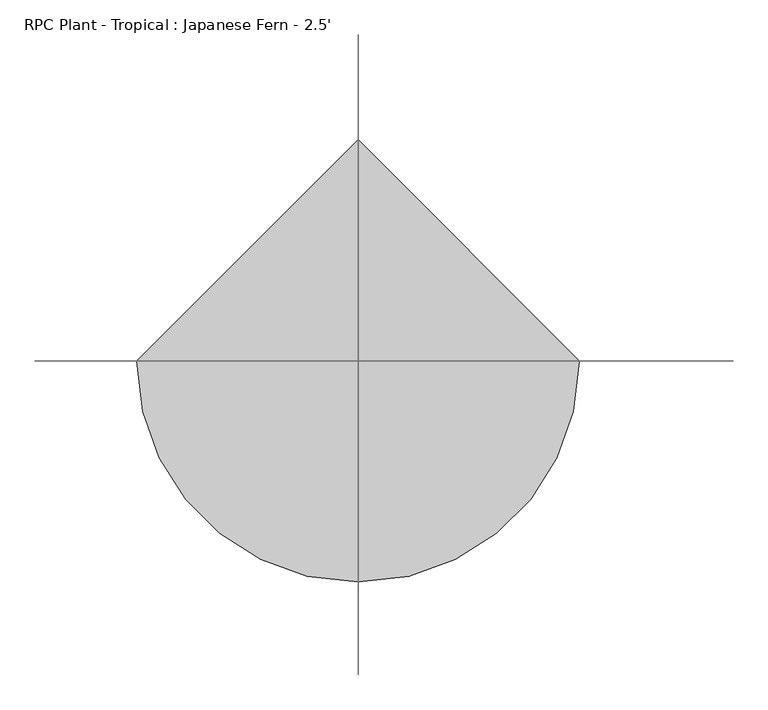
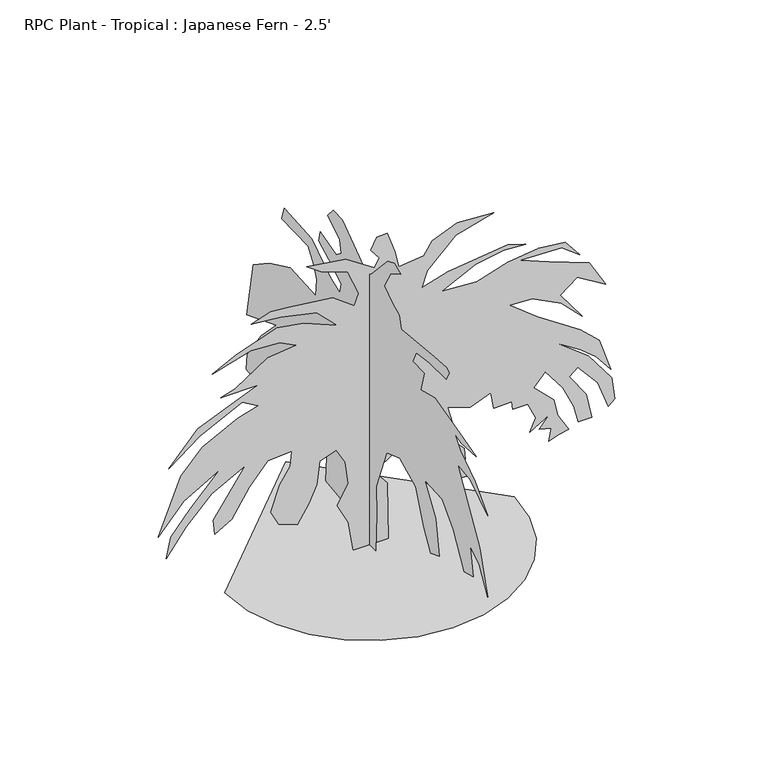
"""IFC4 building model written with IfcOpenShell, lengths in millimetres: geographic element geometry, RPC Plant - Tropical : Japanese Fern - 2.5'."""

from ifc_helpers import new_model, si_unit, origin, place, context, project, spatial, triangles, source, transform, mapped, element, save


def rpc_plant_tropical_japanese_fern_2_5_30b4c15b(model_context):
    return source(origin(), model_context, "Body", "Tessellation", [
        triangles([(-340.212337, 0.0, 2.34e-05), (-331.2181912, -77.9542988, 2.34e-05), (-305.6048564, -149.5428615, 2.34e-05), (-265.4195731, -212.7146324, 2.34e-05), (-212.7146324, -265.4195731, 2.34e-05), (-149.5428615, -305.6048564, 2.34e-05), (-77.9542988, -331.2181912, 2.34e-05), (1.49e-05, -340.212337, 2.34e-05), (77.9542988, -331.2181912, 2.34e-05), (149.5428615, -305.6048564, 2.34e-05), (212.7146324, -265.4195731, 2.34e-05), (265.4195731, -212.7146324, 2.34e-05), (305.6048564, -149.5428615, 2.34e-05), (331.2181912, -77.9542988, 2.34e-05), (340.212337, 2.97e-05, 2.34e-05), (-4.46e-05, 340.212337, 2.34e-05), (-37.8980319, 2.29e-05, 3.6e-06), (-50.0874814, 2.41e-05, 73.5418183), (-75.8826774, 2.22e-05, 123.7339445), (-49.5540792, 1.83e-05, 170.5209506), (-56.979003, 1.53e-05, 225.9335385), (-77.3492758, 1.4e-05, 262.2445852), (-116.2627981, 1.66e-05, 248.3474865), (-123.5028085, 2.02e-05, 192.7652324), (-143.0648503, 2.35e-05, 151.8270789), (-169.0734009, 2.72e-05, 109.3715308), (-213.7047246, 2.81e-05, 126.2541304), (-232.5443813, 2.67e-05, 163.0480237), (-210.7659323, 2.22e-05, 223.3318078), (-185.9735321, 1.89e-05, 260.6164324), (-182.3167059, 1.66e-05, 296.5396212), (-238.5613832, 1.93e-05, 292.8185184), (-282.7321973, 2.42e-05, 242.1521888), (-323.5728004, 2.99e-05, 177.126216), (-363.5396922, 3.3e-05, 153.4968807), (-367.1566226, 3.1e-05, 190.2732333), (-291.3732759, 2.12e-05, 298.3785896), (-370.9310652, 2.72e-05, 256.7835813), (-430.3492407, 3.34e-05, 195.5366293), (-477.8725754, 3.92e-05, 133.2528402), (-467.4636904, 3.58e-05, 182.8625483), (-420.8344145, 3.05e-05, 237.2243282), (-351.5280344, 2.32e-05, 310.1438599), (-436.732245, 2.98e-05, 261.3606638), (-497.0571965, 3.65e-05, 192.7571115), (-443.5089389, 2.62e-05, 326.4709519), (-392.9096655, 2.08e-05, 380.0648827), (-309.8949288, 1.46e-05, 423.094996), (-260.7967811, 1.16e-05, 437.3545544), (-299.3412489, 1.2e-05, 459.500768), (-398.9192914, 1.93e-05, 409.5872812), (-471.8705798, 2.58e-05, 354.6903414), (-403.1941031, 1.83e-05, 430.1180775), (-300.6061608, 1.12e-05, 473.1100754), (-262.5823916, 8.7e-06, 488.4237482), (-349.0058046, 1.24e-05, 488.2357873), (-315.6607106, 1.04e-05, 498.3805169), (-238.5613832, 4e-06, 548.5353044), (-172.4069002, 6e-07, 556.9452561), (-210.7659323, 1.1e-06, 576.3305191), (-278.7875798, 3.9e-06, 580.4732532), (-369.1987945, 9.4e-06, 554.0953574), (-313.0699167, 5.2e-06, 582.9446503), (-216.6861742, -1e-06, 616.0738781), (-154.0988607, -3.1e-06, 605.5227053), (-75.0741966, -4.5e-06, 572.1420393), (-123.4916265, -5.3e-06, 620.6382071), (-209.0953766, -2.7e-06, 638.8728498), (-277.4743968, -1e-07, 645.8171934), (-232.2393309, -3e-06, 661.5423237), (-190.0088236, -4.6e-06, 657.7145777), (-85.7208487, -8.4e-06, 644.6056395), (-35.6564855, -8.3e-06, 606.9044523), (-24.5384073, -1.05e-05, 634.6996307), (-50.8667489, -1.3e-05, 696.1980572), (-113.4009815, -1.16e-05, 718.2401711), (-146.8372491, -1.16e-05, 743.1016623), (-55.5814956, -1.48e-05, 730.2366045), (11.5952668, -1.5e-05, 684.7325506), (23.1518731, -1.68e-05, 706.0913486), (3.2567592, -1.75e-05, 731.9840996), (17.6289544, -1.97e-05, 758.3441912), (41.4979712, -2.09e-05, 760.5615704), (59.6452374, -1.86e-05, 708.9971306), (68.5156716, -1.65e-05, 668.0955574), (127.4710438, -1.95e-05, 674.2321741), (147.7915331, -2.21e-05, 704.1889212), (206.1616894, -2.62e-05, 729.2028013), (292.3257614, -2.96e-05, 723.6452917), (202.8348031, -2.42e-05, 698.6847513), (136.1791696, -1.75e-05, 634.3440565), (123.7575623, -1.46e-05, 595.466851), (183.9252741, -1.84e-05, 615.2432602), (325.6810292, -2.56e-05, 631.9208759), (367.486835, -2.67e-05, 619.3809437), (315.6911957, -2.46e-05, 622.1876038), (249.7079049, -2.1e-05, 609.8203354), (170.7500609, -1.52e-05, 570.6967787), (252.258585, -1.85e-05, 566.1527246), (325.6530876, -2.3e-05, 588.2608592), (397.9490381, -2.68e-05, 598.5656445), (460.1815041, -2.91e-05, 591.0853598), (495.2309272, -2.81e-05, 548.5353044), (452.9501141, -2.81e-05, 580.5189626), (355.0433722, -2.4e-05, 583.2977174), (420.1841635, -2.53e-05, 556.8741122), (516.8336057, -2.73e-05, 520.4505724), (556.2848313, -2.51e-05, 453.460657), (489.3051261, -2.46e-05, 494.41557), (449.4220591, -2.1e-05, 463.6816175), (500.7909802, -1.9e-05, 392.8817239), (450.7580967, -1.98e-05, 442.9146074), (383.0951119, -1.89e-05, 477.7430411), (329.99392, -1.68e-05, 480.9358332), (395.1677399, -1.66e-05, 429.0157465), (495.6652757, -1.69e-05, 361.8734422), (541.06265, -1.64e-05, 319.2167072), (567.5802175, -1.27e-05, 237.3833302), (533.9328526, -1.38e-05, 280.9008592), (497.6007317, -1.4e-05, 310.7127932), (440.194243, -1.36e-05, 346.6664852), (514.6872977, -1.35e-05, 290.0397636), (570.595186, -1.15e-05, 215.9856355), (576.6531012, -8.5e-06, 161.5684811), (561.938883, -7.1e-06, 148.2847988), (536.9249665, -1e-05, 214.9932542), (489.6734176, -1.12e-05, 270.583393), (469.5464848, -9.4e-06, 254.0962635), (510.5775922, -7.7e-06, 195.5264555), (523.0261056, -4.6e-06, 134.3872005), (491.7079591, -3.2e-06, 133.6020922), (481.1339315, -5.3e-06, 176.3159639), (454.7662096, -7.4e-06, 231.6510674), (413.5344604, -8.8e-06, 285.1248746), (386.501263, -5.8e-06, 255.5745526), (434.0830244, -5.2e-06, 209.4342185), (443.1813063, -3e-06, 166.6068182), (468.6523896, -1.6e-06, 123.9640722), (446.3842358, -3e-07, 118.289464), (421.5049404, 1.3e-06, 110.591996), (428.004798, -8e-07, 139.9015351), (399.5416008, 0.0, 147.6790127), (422.9629183, -2.7e-06, 176.0799863), (377.2150203, 9e-07, 148.592647), (391.2256476, -1.5e-06, 179.1531272), (372.9656067, -3.1e-06, 218.8891102), (336.6588839, -1.5e-06, 219.0854463), (334.8783603, -2.6e-06, 238.301043), (292.3257614, -6e-07, 237.2294151), (285.8309907, -2.8e-06, 277.7512695), (236.7361495, 5e-07, 259.4658122), (183.9252741, 1.8e-06, 276.1434461), (200.6023993, 4.7e-06, 214.9932542), (199.418242, 6.4e-06, 187.1818159), (222.8385421, 6.9e-06, 162.1823971), (225.6180599, 8.4e-06, 134.3872005), (208.5548754, 9.9e-06, 121.5754553), (237.8440942, 1.05e-05, 90.4480402), (182.0385615, 1.28e-05, 92.8412262), (191.5158174, 1e-05, 133.3458033), (165.4579784, 1e-05, 152.2179799), (173.5882597, 8.2e-06, 176.3515177), (109.0494575, 1.14e-05, 169.6062899), (94.9809212, 1.06e-05, 192.7571115), (145.0122605, 6.8e-06, 220.5522899), (83.3228392, 9.3e-06, 223.7369429), (11.6764698, 1.52e-05, 177.2189248), (42.170055, 1.61e-05, 139.9462362), (44.9495728, 1.82e-05, 0.0), (0.00212, 26.6938489, 3.6e-06), (0.0021253, 22.2078332, 125.235588), (0.0021271, 60.1697466, 128.8281648), (0.002126, 119.4035039, 42.9622804), (0.0021289, 177.9956579, 51.1230378), (0.0021314, 173.4581986, 113.1355544), (0.0021337, 137.5657583, 202.421547), (0.0021299, 136.57414, 252.5593115), (0.0021317, 167.407932, 262.8744886), (0.0021371, 226.3958104, 190.2732333), (0.0021373, 288.3557457, 133.4656906), (0.0021388, 315.632769, 140.3605096), (0.0021407, 309.8923854, 190.0641981), (0.0021433, 346.6360002, 212.5124464), (0.0021443, 409.4094941, 172.1231784), (0.0021442, 453.2701527, 125.235588), (0.0021466, 501.6723581, 132.7981805), (0.0021481, 497.133391, 172.1231784), (0.0021432, 441.1721629, 252.2857635), (0.0021433, 378.8939512, 316.9053294), (0.0021465, 498.6472157, 270.4360728), (0.0021515, 472.2337844, 410.5144049), (0.0021506, 407.8956694, 453.4479761), (0.0021486, 323.1969149, 492.7747544), (0.0021437, 217.6417118, 487.9487409), (0.0021455, 214.2957677, 530.5851645), (0.0021473, 226.9167634, 559.1017015), (0.0021497, 249.3380874, 591.8626016), (0.0021545, 357.9821463, 594.1105021), (0.0021554, 347.3954378, 625.8731346), (0.0021502, 235.3830889, 618.7560545), (0.0021449, 161.3091401, 570.0389337), (0.0021424, 119.7014417, 554.0699593), (0.0021433, 115.4461873, 579.5537599), (0.0021468, 165.8956152, 609.2361777), (0.0021495, 206.7331843, 630.4121017), (0.0021444, 199.1706008, 657.6358034), (0.0021408, 134.2553771, 640.0184195), (0.0021406, 114.4705746, 656.1245584), (0.0021422, 120.4276329, 685.149095), (0.0021457, 170.4330744, 716.6247173), (0.0021458, 147.7455603, 742.3371014), (0.0021442, 111.4454322, 740.823313), (0.002139, 41.6899925, 691.1155186), (0.0021365, 10.7464246, 665.9695244), (0.0021362, -10.1176737, 680.5009048), (0.0021365, -74.5923583, 749.8987038), (0.0021358, -101.8173226, 761.9992733), (0.0021341, -127.5299701, 749.8987038), (0.0021349, -87.1447716, 726.4240465), (0.002134, -60.7928054, 680.9606152), (0.0021316, -92.5270285, 657.5951809), (0.0021298, -121.8045655, 644.2526087), (0.0021341, -129.7537351, 615.210268), (0.0021228, -265.1681168, 628.8983133), (0.0021208, -315.0816035, 631.9234194), (0.00212, -325.668312, 624.3618896), (0.0021255, -313.5677788, 601.6746117), (0.0021285, -243.6485001, 600.9557965), (0.0021305, -191.8444855, 593.8259992), (0.0021298, -176.5968879, 563.282551), (0.0021277, -223.3409642, 562.4341653), (0.0021262, -209.0156213, 512.3124063), (0.0021243, -266.6794162, 527.5625656), (0.0021188, -366.5470304, 501.9288832), (0.002115, -434.5681692, 482.1855025), (0.0021175, -375.2998755, 480.0595058), (0.002119, -348.4190672, 487.3848581), (0.0021168, -370.0115719, 459.7014462), (0.0021124, -430.801357, 418.7795254), (0.0021078, -482.9678312, 365.7240792), (0.0021129, -410.4102324, 411.3017841), (0.0021154, -360.3773852, 417.8549815), (0.0021108, -398.4519507, 351.1901917), (0.0021049, -449.6938448, 265.8970875), (0.0021049, -481.8349789, 162.1823971), (0.002103, -448.18002, 222.0356478), (0.0021056, -410.473746, 244.4529204), (0.0021022, -423.4226649, 177.6834858), (0.0021093, -387.3318446, 167.7414328), (0.0021087, -342.3053052, 246.2357331), (0.0021128, -296.4634267, 293.7202257), (0.0021161, -226.1207364, 298.3785896), (0.0021111, -271.2183834, 229.5982494), (0.0021128, -284.3374772, 144.5642138), (0.0021137, -249.3695898, 130.0336417), (0.002117, -221.7963819, 179.3619262), (0.002116, -188.1828268, 259.1153067), (0.0021202, -123.9887073, 290.1007337), (0.0021217, -70.0716722, 271.1447323), (0.0021248, -27.498267, 162.3606929), (0.0021217, -30.4360283, 94.6027103), (0.0021177, -25.7012178, 2.43e-05)], [[15, 16, 1], [14, 15, 1], [14, 1, 2], [13, 14, 2], [13, 2, 3], [13, 3, 4], [12, 13, 4], [11, 12, 4], [11, 4, 5], [11, 5, 6], [11, 6, 7], [11, 7, 8], [11, 8, 9], [11, 9, 10], [110, 111, 112], [51, 52, 53], [61, 62, 63], [102, 103, 104], [94, 95, 96], [55, 56, 57], [88, 89, 90], [44, 45, 46], [117, 118, 119], [61, 63, 64], [68, 69, 70], [39, 40, 41], [107, 108, 109], [76, 77, 78], [39, 41, 42], [75, 76, 78], [38, 39, 42], [38, 42, 43], [60, 61, 64], [143, 144, 145], [93, 94, 96], [93, 96, 97], [93, 97, 98], [68, 70, 71], [37, 38, 43], [55, 57, 58], [157, 158, 159], [157, 159, 160], [75, 78, 79], [92, 93, 98], [74, 75, 79], [67, 68, 71], [67, 71, 72], [110, 112, 113], [139, 140, 141], [87, 88, 90], [87, 90, 91], [86, 87, 91], [117, 119, 120], [116, 117, 120], [116, 120, 121], [115, 116, 121], [101, 102, 104], [101, 104, 105], [100, 101, 105], [106, 107, 109], [34, 35, 36], [141, 142, 143], [43, 44, 46], [43, 46, 47], [124, 125, 126], [123, 124, 126], [122, 123, 126], [122, 126, 127], [34, 36, 37], [33, 34, 37], [32, 33, 37], [60, 64, 65], [59, 60, 65], [137, 138, 139], [137, 139, 141], [137, 141, 143], [136, 137, 143], [121, 122, 127], [50, 51, 53], [50, 53, 54], [66, 67, 72], [66, 72, 73], [106, 109, 110], [106, 110, 113], [129, 130, 131], [129, 131, 132], [129, 132, 133], [128, 129, 133], [128, 133, 134], [43, 47, 48], [37, 43, 48], [105, 106, 113], [105, 113, 114], [100, 105, 114], [99, 100, 114], [59, 65, 66], [163, 164, 165], [162, 163, 165], [168, 169, 17], [168, 17, 18], [168, 18, 19], [168, 19, 20], [167, 168, 20], [167, 20, 21], [146, 147, 148], [121, 127, 128], [121, 128, 134], [85, 86, 91], [148, 149, 150], [37, 48, 49], [32, 37, 49], [31, 32, 49], [85, 91, 92], [25, 26, 27], [25, 27, 28], [25, 28, 29], [24, 25, 29], [24, 29, 30], [23, 24, 30], [23, 30, 31], [136, 143, 145], [135, 136, 145], [135, 145, 146], [135, 146, 148], [82, 83, 84], [81, 82, 84], [80, 81, 84], [80, 84, 85], [79, 80, 85], [50, 54, 55], [49, 50, 55], [160, 161, 162], [156, 157, 160], [155, 156, 160], [155, 160, 162], [154, 155, 162], [154, 162, 165], [153, 154, 165], [152, 153, 165], [74, 79, 85], [74, 85, 92], [73, 74, 92], [166, 167, 21], [55, 58, 59], [166, 21, 22], [152, 165, 166], [135, 148, 150], [134, 135, 150], [121, 134, 150], [115, 121, 150], [114, 115, 150], [114, 150, 151], [114, 151, 152], [99, 114, 152], [98, 99, 152], [98, 152, 166], [98, 166, 22], [92, 98, 22], [73, 92, 22], [66, 73, 22], [59, 66, 22], [55, 59, 22], [49, 55, 22], [31, 49, 22], [23, 31, 22], [244, 245, 246], [239, 240, 241], [234, 235, 236], [234, 236, 237], [233, 234, 237], [238, 239, 241], [238, 241, 242], [217, 218, 219], [216, 217, 219], [189, 190, 191], [244, 246, 247], [215, 216, 219], [215, 219, 220], [197, 198, 199], [197, 199, 200], [230, 231, 232], [189, 191, 192], [209, 210, 211], [209, 211, 212], [209, 212, 213], [208, 209, 213], [197, 200, 201], [196, 197, 201], [195, 196, 201], [243, 244, 247], [262, 170, 171], [261, 262, 171], [260, 261, 171], [205, 206, 207], [204, 205, 207], [203, 204, 207], [185, 186, 187], [184, 185, 187], [184, 187, 188], [183, 184, 188], [183, 188, 189], [173, 174, 175], [172, 173, 175], [172, 175, 176], [247, 248, 249], [247, 249, 250], [243, 247, 250], [243, 250, 251], [242, 243, 251], [254, 255, 256], [253, 254, 256], [253, 256, 257], [252, 253, 257], [225, 226, 227], [224, 225, 227], [224, 227, 228], [223, 224, 228], [223, 228, 229], [223, 229, 230], [180, 181, 182], [179, 180, 182], [189, 192, 193], [189, 193, 194], [252, 257, 258], [203, 207, 208], [242, 251, 252], [208, 213, 214], [203, 208, 214], [183, 189, 194], [182, 183, 194], [179, 182, 194], [178, 179, 194], [177, 178, 194], [195, 201, 202], [194, 195, 202], [177, 194, 202], [237, 238, 242], [237, 242, 252], [233, 237, 252], [232, 233, 252], [232, 252, 258], [230, 232, 258], [230, 258, 259], [223, 230, 259], [221, 222, 223], [221, 223, 259], [220, 221, 259], [215, 220, 259], [214, 215, 259], [203, 214, 259], [202, 203, 259], [177, 202, 259], [177, 259, 260], [176, 177, 260], [172, 176, 260], [172, 260, 171]], closed=False),
    ])


if __name__ == "__main__":
    model = new_model("IFC4")
    model_context = context("Model", 3, world=origin())
    ifc_project = project(units=[si_unit("LENGTHUNIT", "METRE", prefix="MILLI")], contexts=[model_context])
    site = spatial("IfcSite", under=ifc_project)
    building = spatial("IfcBuilding", under=site)
    placement = place(None, origin())
    rpc_plant_tropical_japanese_fern_2_5_shape = rpc_plant_tropical_japanese_fern_2_5_30b4c15b(model_context)
    element("IfcGeographicElement", 1, ObjectType="RPC Plant - Tropical : Japanese Fern - 2.5'", at=placement, inside=building, context=model_context, shape_type="MappedRepresentation", body=[
        mapped(rpc_plant_tropical_japanese_fern_2_5_shape, transform((0.0, 0.0, 0.0), x_axis=(1.0, 0.0, 0.0), y_axis=(0.0, 1.0, 0.0), z_axis=(0.0, 0.0, 1.0))),
    ])
    save(model, "model.ifc")

# Revit data of these elements
# Type "RPC Plant - Tropical : Japanese Fern - 2.5'"
#   built-in parameter 1005198 = "{2, 15},{39, RPC-16-G1GK-JAPX-7J4P-Q000-ST1L-LVER-AU},{1, 0},{1, 0},{2, 13},{1, 8},{5, Color},{1, 0},{1, 0},{3, 0.8},{3, 0.8},{3, 0.8},{1, 8},{7, BBoxMin},{1, 0},{1, 0},{1, 0},{1, 0},{1, 0},{1, 8},{7, BBoxMax},{1, 0},{1, 0},{1, 0},{1, 0},{1, 0},{2, 11},{9, RPCTypeId},{1, 0},{1, 0},{39, RPC-16-G1GK-JAPX-7J4P-Q000-ST1L-LVER-AU},{1, 6},{14, RPCPlantHeight},{1, 0},{1, 0},{3, 2.5},{2, 11},{7, keyword},{1, 0},{1, 0},{35, :RPCs:Shrubs [General]:Geometry:RPC},{2, 11},{8, category},{1, 0},{1, 0},{16, Shrubs [General]},{2, 11},{12, LocalizedUID},{1, 0},{1, 0},{13, Japanese Fern},{2, 14},{6, Height},{1, 0},{1, 0},{3, 2.5},{1, 2},{16, Cast Reflections},{1, 0},{1, 0},{1, 0},{1, 2},{12, Cast Shadows},{1, 0},{1, 0},{1, 1},{1, 2},{9, Lock View},{1, 0},{1, 0},{1, 0},{1, 4},{5, ViewC},{1, 0},{1, 0},{1, 0},{21, assetlibrary_base.fbx},{1, 5},"
#   built-in parameter 1005195 = "RPC-16-G1GK-JAPX-7J4P-Q000-ST1L-LVER-AU"
#   Type Comments = "Japanese Fern"
#   Assembly Code = "G2050500"
#   Height = 2' - 6"
#   Default Elevation = 0
